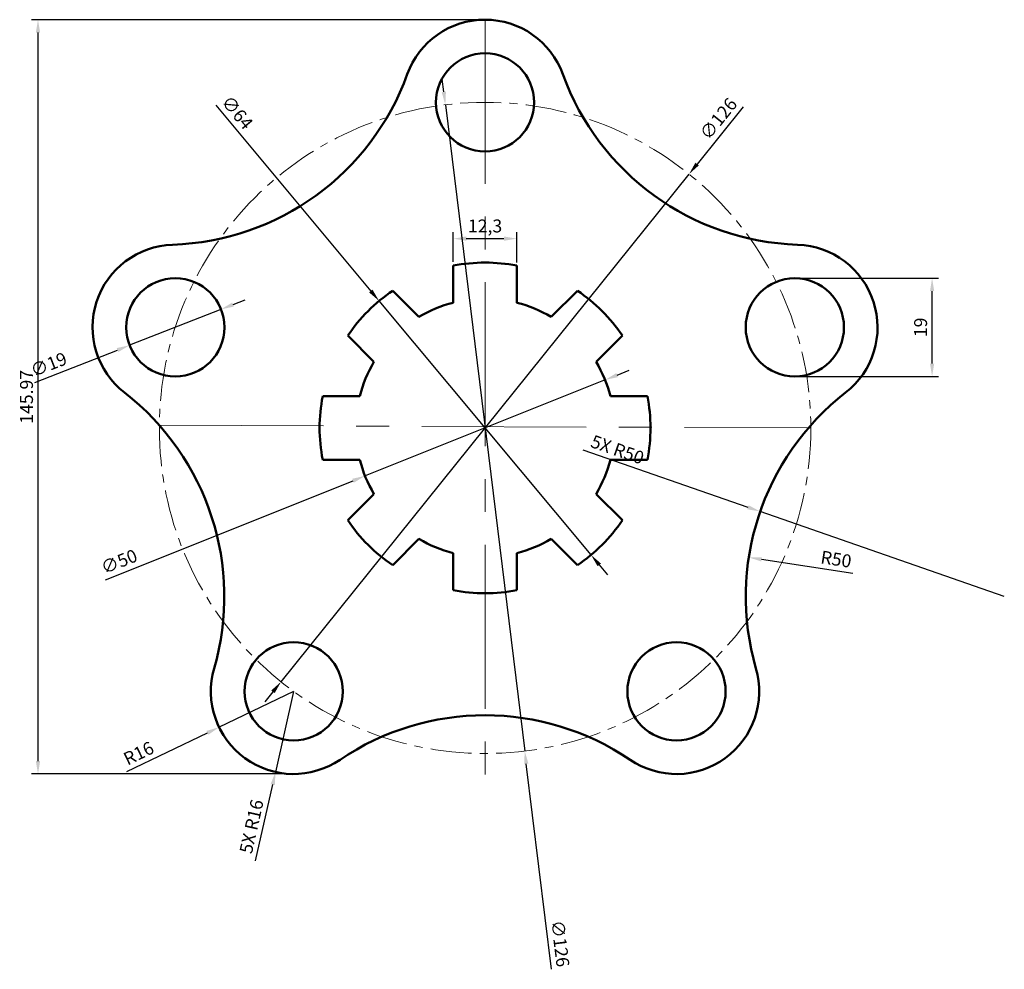
# Model space of a CAD drawing. Units: millimetres. Extents: x 3048 to 3238, y 1408 to 1592.
import ezdxf

# ---------------------------------------------------------------- set-up
doc = ezdxf.new("R2010")
doc.units = ezdxf.units.MM
doc.linetypes.add('CENTER', pattern=[50.8, 31.75, -6.35, 6.35, -6.35])
for name, color, linetype, lineweight in [('M-CNTR', 4, 'CENTER', 18), ('M-DIMS', 2, 'Continuous', 25), ('M-OUTL', 7, 'Continuous', 50)]:
    doc.layers.add(name, color=color, linetype=linetype, lineweight=lineweight)
doc.styles.get("Standard").update_dxf_attribs({"font": 'arial.ttf'})
doc.dimstyles.new('ISO-25', dxfattribs={"dimtxt": 2.5, "dimasz": 2.5, "dimexe": 1.25, "dimexo": 0.625, "dimtad": 1, "dimtxsty": 'Standard', "dimcen": 2.5, "dimadec": 0, "dimazin": 0, "dimtfac": 1, "dimtmove": 0, "dimatfit": 3, "dimfxl": 1, "dimarcsym": 0})

# ---------------------------------------------------------------- blocks, each defined once
blk = doc.blocks.new('*U1')
blk.add_circle((0, 0), 9.5)
blk = doc.blocks.new('*U2')
at = {"layer": 'M-OUTL', "color": 0, "linetype": 'ByBlock', "lineweight": -2, "transparency": 16777216}
blk.add_blockref('*U1', (3137.54, 1575.62), dxfattribs=at)
for p, rotation in [((3077.62, 1532.09), 72), ((3197.45, 1532.09), 287.9999999999999), ((3100.51, 1461.65), 144), ((3174.57, 1461.65), 216)]:
    blk.add_blockref('*U1', p, dxfattribs=dict(at, rotation=rotation))
blk = doc.blocks.new('*D3')
at = {"layer": 'Defpoints', "color": 0, "transparency": 16777216}
for p in [(3143.69, 1549.25), (3131.39, 1544.14), (3143.69, 1544.03)]:
    blk.add_point(p, dxfattribs=at)
at = {"layer": 'M-DIMS', "color": 0, "lineweight": -2, "transparency": 16777216}
for p, q in [((3131.39, 1544.77), (3131.39, 1550.5)), ((3143.69, 1544.65), (3143.69, 1550.5)), ((3133.89, 1549.25), (3141.19, 1549.25))]:
    blk.add_line(p, q, dxfattribs=at)
at = {"layer": 'M-DIMS', "color": 0, "transparency": 16777216}
for points in [[(3133.89, 1549.67), (3133.89, 1548.84), (3131.39, 1549.25)], [(3141.19, 1549.67), (3141.19, 1548.84), (3143.69, 1549.25)]]:
    blk.add_solid(points, dxfattribs=at)
at = {"layer": 'M-DIMS', "color": 0, "transparency": 16777216, "insert": (3137.54, 1551.38), "char_height": 2.5, "attachment_point": 5}
blk.add_mtext('12,3', dxfattribs=at)
blk = doc.blocks.new('*D4')
at = {"layer": 'Defpoints', "color": 0, "transparency": 16777216}
for p in [(3100.51, 1461.65), (3086.09, 1454.71)]:
    blk.add_point(p, dxfattribs=at)
at = {"layer": 'M-DIMS', "color": 0, "lineweight": -2, "transparency": 16777216}
for p, q in [((3100.51, 1461.65), (3086.09, 1454.71)), ((3068.25, 1446.11), (3083.84, 1453.62))]:
    blk.add_line(p, q, dxfattribs=at)
at = {"layer": 'M-DIMS', "color": 0, "transparency": 16777216}
blk.add_solid([(3083.66, 1454), (3084.02, 1453.25), (3086.09, 1454.71)], dxfattribs=at)
at = {"layer": 'M-DIMS', "color": 0, "transparency": 16777216, "insert": (3070.67, 1449.39), "char_height": 2.5, "attachment_point": 5, "rotation": 25.7312}
blk.add_mtext('R16', dxfattribs=at)
blk = doc.blocks.new('*D5')
at = {"layer": 'Defpoints', "color": 0, "transparency": 16777216}
for p in [(3188.55, 1487.57), (3237.97, 1479.99)]:
    blk.add_point(p, dxfattribs=at)
at = {"layer": 'M-DIMS', "color": 0, "lineweight": -2, "transparency": 16777216}
blk.add_line((3208.67, 1484.48), (3191.02, 1487.19), dxfattribs=at)
at = {"layer": 'M-DIMS', "color": 0, "transparency": 16777216}
blk.add_solid([(3191.08, 1487.6), (3190.96, 1486.78), (3188.55, 1487.57)], dxfattribs=at)
at = {"layer": 'M-DIMS', "color": 0, "transparency": 16777216, "insert": (3205.39, 1486.91), "char_height": 2.5, "attachment_point": 5, "rotation": 351.2796}
blk.add_mtext('R50', dxfattribs=at)
blk = doc.blocks.new('*D6')
at = {"layer": 'Defpoints', "color": 0, "transparency": 16777216}
for p in [(3176.99, 1561.74), (3098.08, 1463.51)]:
    blk.add_point(p, dxfattribs=at)
at = {"layer": 'M-DIMS', "color": 0, "lineweight": -2, "transparency": 16777216}
for p, q in [((3187.43, 1574.73), (3178.56, 1563.69)), ((3098.08, 1463.51), (3176.99, 1561.74)), ((3096.52, 1461.56), (3094.95, 1459.61))]:
    blk.add_line(p, q, dxfattribs=at)
at = {"layer": 'M-DIMS', "color": 0, "transparency": 16777216}
for points in [[(3178.23, 1563.95), (3178.88, 1563.43), (3176.99, 1561.74)], [(3096.19, 1461.82), (3096.84, 1461.3), (3098.08, 1463.51)]]:
    blk.add_solid(points, dxfattribs=at)
at = {"layer": 'M-DIMS', "color": 0, "transparency": 16777216, "insert": (3182.92, 1572.26), "char_height": 2.5, "attachment_point": 5, "rotation": 51.2249}
blk.add_mtext('∅126', dxfattribs=at)
blk = doc.blocks.new('*D7')
at = {"layer": 'Defpoints', "color": 0, "transparency": 16777216}
for p in [(3086.46, 1535.57), (3068.78, 1528.61)]:
    blk.add_point(p, dxfattribs=at)
at = {"layer": 'M-DIMS', "color": 0, "lineweight": -2, "transparency": 16777216}
for p, q in [((3088.79, 1536.49), (3091.11, 1537.4)), ((3086.46, 1535.57), (3068.78, 1528.61)), ((3050.46, 1521.39), (3066.45, 1527.69))]:
    blk.add_line(p, q, dxfattribs=at)
at = {"layer": 'M-DIMS', "color": 0, "transparency": 16777216}
for points in [[(3088.63, 1536.88), (3088.94, 1536.1), (3086.46, 1535.57)], [(3066.3, 1528.08), (3066.61, 1527.31), (3068.78, 1528.61)]]:
    blk.add_solid(points, dxfattribs=at)
at = {"layer": 'M-DIMS', "color": 0, "transparency": 16777216, "insert": (3053.25, 1524.61), "char_height": 2.5, "attachment_point": 5, "rotation": 21.4945}
blk.add_mtext('∅19', dxfattribs=at)
blk = doc.blocks.new('*D8')
at = {"layer": 'Defpoints', "color": 0, "transparency": 16777216}
for p in [(3117.04, 1537.2), (3158.03, 1488.05)]:
    blk.add_point(p, dxfattribs=at)
at = {"layer": 'M-DIMS', "color": 0, "lineweight": -2, "transparency": 16777216}
for p, q in [((3085.44, 1575.09), (3115.44, 1539.12)), ((3158.03, 1488.05), (3117.04, 1537.2)), ((3159.63, 1486.13), (3161.23, 1484.21))]:
    blk.add_line(p, q, dxfattribs=at)
at = {"layer": 'M-DIMS', "color": 0, "transparency": 16777216}
for points in [[(3115.76, 1539.39), (3115.12, 1538.85), (3117.04, 1537.2)], [(3159.95, 1486.39), (3159.31, 1485.86), (3158.03, 1488.05)]]:
    blk.add_solid(points, dxfattribs=at)
at = {"layer": 'M-DIMS', "color": 0, "transparency": 16777216, "insert": (3089.37, 1573.46), "char_height": 2.5, "attachment_point": 5, "rotation": 309.8239}
blk.add_mtext('∅64', dxfattribs=at)
blk = doc.blocks.new('*D9')
at = {"layer": 'Defpoints', "color": 0, "transparency": 16777216}
for p in [(3160.75, 1521.91), (3114.33, 1503.34)]:
    blk.add_point(p, dxfattribs=at)
at = {"layer": 'M-DIMS', "color": 0, "lineweight": -2, "transparency": 16777216}
for p, q in [((3163.07, 1522.84), (3165.39, 1523.77)), ((3160.75, 1521.91), (3114.33, 1503.34)), ((3064.1, 1483.24), (3112, 1502.41))]:
    blk.add_line(p, q, dxfattribs=at)
at = {"layer": 'M-DIMS', "color": 0, "transparency": 16777216}
for points in [[(3162.91, 1523.22), (3163.22, 1522.45), (3160.75, 1521.91)], [(3111.85, 1502.79), (3112.16, 1502.02), (3114.33, 1503.34)]]:
    blk.add_solid(points, dxfattribs=at)
at = {"layer": 'M-DIMS', "color": 0, "transparency": 16777216, "insert": (3066.87, 1486.47), "char_height": 2.5, "attachment_point": 5, "rotation": 21.8063}
blk.add_mtext('∅50', dxfattribs=at)
blk = doc.blocks.new('*D10')
at = {"layer": 'Defpoints', "color": 0, "transparency": 16777216}
for p in [(3051.07, 1591.62), (3137.54, 1591.62), (3100.25, 1445.66)]:
    blk.add_point(p, dxfattribs=at)
at = {"layer": 'M-DIMS', "color": 0, "lineweight": -2, "transparency": 16777216}
for p, q in [((3136.91, 1591.62), (3049.82, 1591.62)), ((3051.07, 1448.16), (3051.07, 1589.12)), ((3099.62, 1445.66), (3049.82, 1445.66))]:
    blk.add_line(p, q, dxfattribs=at)
at = {"layer": 'M-DIMS', "color": 0, "transparency": 16777216}
for points in [[(3050.65, 1589.12), (3051.49, 1589.12), (3051.07, 1591.62)], [(3050.65, 1448.16), (3051.49, 1448.16), (3051.07, 1445.66)]]:
    blk.add_solid(points, dxfattribs=at)
at = {"layer": 'M-DIMS', "color": 0, "transparency": 16777216, "insert": (3049.17, 1518.64), "char_height": 2.5, "attachment_point": 5, "rotation": 90}
blk.add_mtext('145.97', dxfattribs=at)
blk = doc.blocks.new('*D11')
at = {"layer": 'Defpoints', "color": 0, "transparency": 16777216}
for p in [(3197.45, 1541.59), (3224, 1541.59), (3197.45, 1522.59)]:
    blk.add_point(p, dxfattribs=at)
at = {"layer": 'M-DIMS', "color": 0, "lineweight": -2, "transparency": 16777216}
for p, q in [((3198.08, 1541.59), (3225.25, 1541.59)), ((3224, 1525.09), (3224, 1539.09)), ((3198.08, 1522.59), (3225.25, 1522.59))]:
    blk.add_line(p, q, dxfattribs=at)
at = {"layer": 'M-DIMS', "color": 0, "transparency": 16777216}
for points in [[(3223.59, 1539.09), (3224.42, 1539.09), (3224, 1541.59)], [(3223.59, 1525.09), (3224.42, 1525.09), (3224, 1522.59)]]:
    blk.add_solid(points, dxfattribs=at)
at = {"layer": 'M-DIMS', "color": 0, "transparency": 16777216, "insert": (3222.1, 1532.09), "char_height": 2.5, "attachment_point": 5, "rotation": 90}
blk.add_mtext('19', dxfattribs=at)
blk = doc.blocks.new('*D12')
at = {"layer": 'Defpoints', "color": 0, "transparency": 16777216}
for p in [(3129.86, 1575.15), (3145.21, 1450.09)]:
    blk.add_point(p, dxfattribs=at)
at = {"layer": 'M-DIMS', "color": 0, "lineweight": -2, "transparency": 16777216}
for p, q in [((3129.56, 1577.63), (3129.25, 1580.12)), ((3129.86, 1575.15), (3145.21, 1450.09)), ((3150.39, 1407.86), (3145.51, 1447.61))]:
    blk.add_line(p, q, dxfattribs=at)
at = {"layer": 'M-DIMS', "color": 0, "transparency": 16777216}
for points in [[(3129.97, 1577.69), (3129.15, 1577.58), (3129.86, 1575.15)], [(3145.93, 1447.66), (3145.1, 1447.56), (3145.21, 1450.09)]]:
    blk.add_solid(points, dxfattribs=at)
at = {"layer": 'M-DIMS', "color": 0, "transparency": 16777216, "insert": (3151.77, 1412.81), "char_height": 2.5, "attachment_point": 5, "rotation": 276.9957}
blk.add_mtext('∅126', dxfattribs=at)
blk = doc.blocks.new('*D13')
at = {"layer": 'Defpoints', "color": 0, "transparency": 16777216}
for p in [(3100.51, 1461.65), (3097.01, 1446.04)]:
    blk.add_point(p, dxfattribs=at)
at = {"layer": 'M-DIMS', "color": 0, "lineweight": -2, "transparency": 16777216}
for p, q in [((3100.51, 1461.65), (3097.01, 1446.04)), ((3093.16, 1428.87), (3096.46, 1443.6))]:
    blk.add_line(p, q, dxfattribs=at)
at = {"layer": 'M-DIMS', "color": 0, "transparency": 16777216}
blk.add_solid([(3096.05, 1443.69), (3096.87, 1443.51), (3097.01, 1446.04)], dxfattribs=at)
at = {"layer": 'M-DIMS', "color": 0, "transparency": 16777216, "insert": (3092.68, 1435.43), "char_height": 2.5, "attachment_point": 5, "rotation": 77.3674}
blk.add_mtext('5X R16', dxfattribs=at)
blk = doc.blocks.new('*D14')
at = {"layer": 'Defpoints', "color": 0, "transparency": 16777216}
for p in [(3190.75, 1496.45), (3237.97, 1479.99)]:
    blk.add_point(p, dxfattribs=at)
at = {"layer": 'M-DIMS', "color": 0, "lineweight": -2, "transparency": 16777216}
for p, q in [((3156.48, 1508.39), (3188.39, 1497.27)), ((3237.97, 1479.99), (3190.75, 1496.45))]:
    blk.add_line(p, q, dxfattribs=at)
at = {"layer": 'M-DIMS', "color": 0, "transparency": 16777216}
blk.add_solid([(3188.53, 1497.66), (3188.26, 1496.88), (3190.75, 1496.45)], dxfattribs=at)
at = {"layer": 'M-DIMS', "color": 0, "transparency": 16777216, "insert": (3163.05, 1508.12), "char_height": 2.5, "attachment_point": 5, "rotation": 340.7846}
blk.add_mtext('5X R50', dxfattribs=at)

msp = doc.modelspace()

# ---------------------------------------------------------------- linework, layer by layer
at = {"layer": 'M-CNTR', "transparency": 33554534}
for p, q in [((3137.537, 1591.623), (3137.537, 1444.322)), ((3074.539, 1513.136), (3200.537, 1512.623))]:
    msp.add_line(p, q, dxfattribs=at)
at = {"layer": 'M-CNTR'}
for p, q in [((3074.987, 1512.623), (3074.537, 1512.623)), ((3200.086, 1512.623), (3200.537, 1512.623))]:
    msp.add_line(p, q, dxfattribs=at)
at = {"layer": 'M-CNTR', "ltscale": 0.25, "transparency": 33554534}
msp.add_circle((3137.537, 1512.623), 63, dxfattribs=at)
at = {"layer": 'M-OUTL'}
for p, q in [((3131.387, 1536.854), (3131.387, 1544.026)), ((3143.687, 1536.854), (3143.687, 1544.026)), ((3124.751, 1534.106), (3119.68, 1539.177)), ((3150.322, 1534.106), (3155.394, 1539.177)), ((3116.054, 1525.408), (3110.982, 1530.479)), ((3159.02, 1525.408), (3164.091, 1530.479)), ((3113.305, 1518.773), (3106.133, 1518.773)), ((3161.769, 1518.773), (3168.94, 1518.773)), ((3113.305, 1506.473), (3106.133, 1506.473)), ((3161.769, 1506.473), (3168.94, 1506.473)), ((3116.054, 1499.837), (3110.982, 1494.766)), ((3159.02, 1499.837), (3164.091, 1494.766)), ((3124.751, 1491.139), (3119.68, 1486.068)), ((3150.322, 1491.139), (3155.394, 1486.068)), ((3131.387, 1481.219), (3131.387, 1488.391)), ((3143.687, 1481.219), (3143.687, 1488.391))]:
    msp.add_line(p, q, dxfattribs=at)
for centre, radius, start, end in [((3137.537, 1575.623), 16, 19.87033, 160.12967), ((3075.466, 1598.055), 50, 271.87033, 340.12967), ((3199.607, 1598.055), 50, 199.87033, 268.12967), ((3077.62, 1532.091), 16, 91.87033, 232.12967), ((3197.453, 1532.091), 16, 307.87033, 88.12967), ((3137.537, 1512.623), 32, 78.91953, 101.08047), ((3137.537, 1512.623), 32, 123.91953, 146.08047), ((3137.537, 1512.623), 32, 33.91953, 56.08047), ((3137.537, 1512.623), 25, 104.24094, 120.75906), ((3137.537, 1512.623), 25, 59.24094, 75.75906), ((3137.537, 1512.623), 25, 149.24094, 165.75906), ((3137.537, 1512.623), 25, 14.24094, 30.75906), ((3037.104, 1479.99), 50, 343.87033, 52.12967), ((3137.537, 1512.623), 32, 168.91953, 191.08047), ((3137.537, 1512.623), 32, 348.91953, 11.08047), ((3237.969, 1479.99), 50, 127.87033, 196.12967), ((3137.537, 1512.623), 25, 194.24094, 210.75906), ((3137.537, 1512.623), 25, 329.24094, 345.75906), ((3137.537, 1512.623), 32, 213.91953, 236.08047), ((3137.537, 1512.623), 32, 303.91953, 326.08047), ((3137.537, 1512.623), 25, 239.24094, 255.75906), ((3137.537, 1512.623), 25, 284.24094, 300.75906), ((3137.537, 1512.623), 32, 258.91953, 281.08047), ((3100.506, 1461.654), 16, 163.87033, 304.12967), ((3174.567, 1461.654), 16, 235.87033, 16.12967), ((3137.537, 1407.022), 50, 55.87033, 124.12967)]:
    msp.add_arc(centre, radius, start, end, dxfattribs=at)

# ---------------------------------------------------------------- block references
msp.add_blockref('*U2', (0, 0), dxfattribs=at)

# ---------------------------------------------------------------- dimensions: what is measured, and where the dimension line sits
at = {"layer": 'M-DIMS'}
for base, p1, p2, override, picture, middle in [((3051.069, 1591.623), (3100.245, 1445.657), (3137.537, 1591.623), {"dimdec": 2, "dimlfac": 1, "dimrnd": 0, "dimzin": 0, "dimdsep": 46, "dimlunit": 2}, '*D10', (3049.168, 1518.64)), ((3224.004, 1541.591), (3197.453, 1522.591), (3197.453, 1541.591), {"dimdec": 0, "dimlfac": 1, "dimrnd": 0, "dimzin": 0, "dimdsep": 46, "dimlunit": 2}, '*D11', (3222.103, 1532.091))]:
    dim = msp.add_linear_dim(base=base, p1=p1, p2=p2, angle=90, dimstyle='ISO-25', override=override, dxfattribs=at)
    dim.commit()
    dim.dimension.update_dxf_attribs({"geometry": picture, "text_midpoint": middle})
for p1, p2, override, picture, middle in [((3129.864, 1575.154), (3145.21, 1450.092), {"dimdec": 0, "dimlfac": 1, "dimrnd": 0, "dimzin": 0, "dimdsep": 46, "dimlunit": 2}, '*D12', (3149.814, 1412.573)), ((3158.031, 1488.046), (3117.043, 1537.199), {"dimclrd": 0, "dimclre": 0, "dimclrt": 0}, '*D8', (3087.859, 1572.198)), ((3098.082, 1463.507), (3176.992, 1561.738), {"dimclrd": 0, "dimclre": 0, "dimclrt": 0}, '*D6', (3184.456, 1571.03)), ((3086.46, 1535.572), (3068.781, 1528.61), {"dimclrd": 0, "dimclre": 0, "dimclrt": 0}, '*D7', (3053.971, 1522.778)), ((3160.748, 1521.909), (3114.326, 1503.336), {"dimclrd": 0, "dimclre": 0, "dimclrt": 0}, '*D9', (3067.604, 1484.643))]:
    dim = msp.add_diameter_dim_2p(p1=p1, p2=p2, dimstyle='ISO-25', override=override, dxfattribs=at)
    dim.commit()
    dim.dimension.update_dxf_attribs({"geometry": picture, "text_midpoint": middle, "dimtype": 163})
dim = msp.add_linear_dim(base=(3143.687, 1549.254), p1=(3131.387, 1544.141), p2=(3143.687, 1544.026), dimstyle='ISO-25', override={"dimclrd": 0, "dimclre": 0, "dimclrt": 0}, dxfattribs=at)
dim.commit()
dim.dimension.update_dxf_attribs({"geometry": '*D3', "text_midpoint": (3137.537, 1551.381)})
dim = msp.add_radius_dim(center=(3237.969, 1479.99), mpoint=(3190.755, 1496.446), text='5X <>', dimstyle='ISO-25', override={"dimdec": 0, "dimlfac": 1, "dimrnd": 0, "dimzin": 0, "dimdsep": 46, "dimlunit": 2}, dxfattribs=at)
dim.commit()
dim.dimension.update_dxf_attribs({"geometry": '*D14', "text_midpoint": (3162.426, 1506.32), "dimtype": 164})
for center, mpoint, picture, middle in [((3237.969, 1479.99), (3188.547, 1487.571), '*D5', (3205.1, 1485.032)), ((3100.506, 1461.654), (3086.093, 1454.708), '*D4', (3071.499, 1447.675))]:
    dim = msp.add_radius_dim(center=center, mpoint=mpoint, dimstyle='ISO-25', override={"dimclrd": 0, "dimclre": 0, "dimclrt": 0}, dxfattribs=at)
    dim.commit()
    dim.dimension.update_dxf_attribs({"geometry": picture, "text_midpoint": middle, "dimtype": 164})
dim = msp.add_radius_dim(center=(3100.506, 1461.654), mpoint=(3097.007, 1446.042), text='5X <>', dimstyle='ISO-25', override={"dimdec": 0, "dimlfac": 1, "dimrnd": 0, "dimzin": 0, "dimdsep": 46, "dimlunit": 2}, dxfattribs=at)
dim.commit()
dim.dimension.update_dxf_attribs({"geometry": '*D13', "text_midpoint": (3092.681, 1435.434)})

doc.saveas('drawing.dxf')
